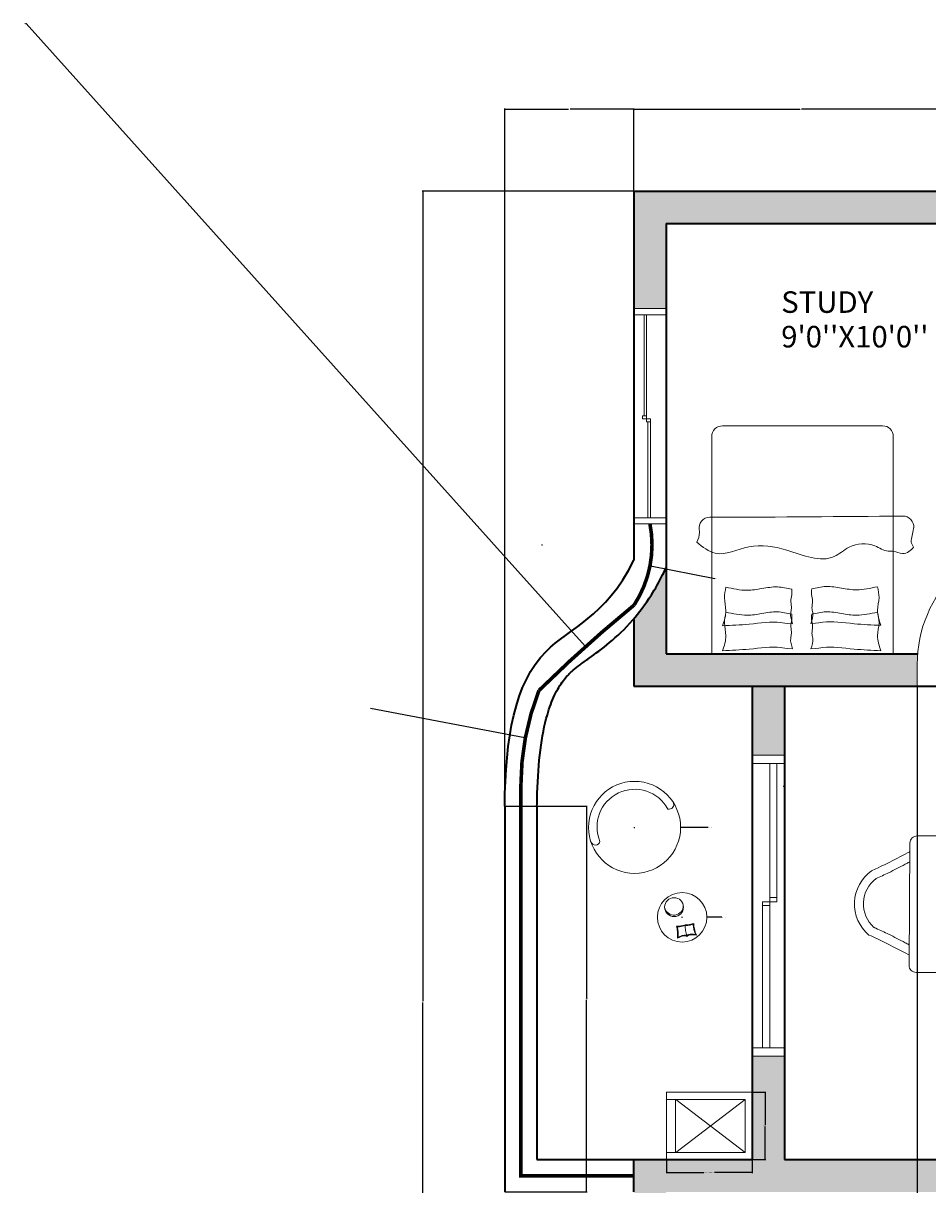
# Model space of a CAD drawing. Units: inches. Extents: x 1789 to 2841, y 3180 to 3702.
# Tile 2 of 14: x 1789 to 2041, y 3378 to 3702. Entities that reach past the tile are written whole.
import ezdxf

# ---------------------------------------------------------------- set-up
doc = ezdxf.new("R2010")
doc.units = ezdxf.units.IN
doc.header["$MEASUREMENT"] = 0
for name, color, linetype, lineweight in [('A-ANNO-DIMS', 2, 'Continuous', 18), ('A-AREA-IDEN', 7, 'Continuous', 18), ('A-FLOR-HRAL', 40, 'Continuous', 18), ('A-WALL', 40, 'Continuous', 35), ('A-WALL-PATT', 252, 'Continuous', 13), ('DORS', 70, 'Continuous', 18), ('FURNITURE', 34, 'Continuous', 18), ('WINDOWS', 130, 'Continuous', 18)]:
    doc.layers.add(name, color=color, linetype=linetype, lineweight=lineweight)
doc.styles.get("Standard").update_dxf_attribs({"font": 'arial.ttf'})
doc.dimstyles.get("Standard").update_dxf_attribs({"dimtxt": 0.18, "dimasz": 0.18, "dimexe": 0.18, "dimexo": 0.0625, "dimgap": 0.09, "dimtad": 0, "dimtih": 1, "dimtoh": 1, "dimdec": 0, "dimzin": 0, "dimdsep": 46, "dimlunit": 3, "dimtxsty": 'Standard', "dimcen": 0.09, "dimadec": 0, "dimazin": 0, "dimtfac": 1, "dimtdec": 0, "dimtofl": 0, "dimtmove": 0, "dimatfit": 3, "dimfxl": 1, "dimtolj": 1, "dimtzin": 0, "dimarcsym": 0})

# ---------------------------------------------------------------- blocks, each defined once
blk = doc.blocks.new('HYJ')
for p, q in [((2206.12, 3649.67), (2234.3, 3649.67)), ((2236.02, 3650.77), (2262.74, 3650.77)), ((2236.02, 3650.11), (2262.74, 3650.11)), ((2206.12, 3649), (2234.3, 3649))]:
    blk.add_line(p, q)
for points in [[(2204.43, 3646.16), (2264.43, 3646.16), (2264.43, 3655.16), (2204.43, 3655.16)], [(2204.43, 3655.16), (2206.12, 3655.16), (2206.12, 3646.16), (2204.43, 3646.16)], [(2264.43, 3655.16), (2262.74, 3655.16), (2262.74, 3646.16), (2264.43, 3646.16)], [(2234.3, 3649.67), (2235.16, 3649.67), (2235.16, 3648.56), (2234.3, 3648.56)], [(2235.16, 3650.77), (2236.02, 3650.77), (2236.02, 3649.67), (2235.16, 3649.67)]]:
    blk.add_lwpolyline(points, close=True)
blk = doc.blocks.new('BED')
blk.add_lwpolyline([(1986.04, 3526.16), (2036.66, 3526.16), (2036.66, 3586.73, 0.414214), (2033.66, 3589.73), (1989.04, 3589.73, 0.414214), (1986.04, 3586.73)], format="xyb", close=True)
for centre, start, end in [((1985.49, 3561.26), 90.0009, 190.5913), ((2039.35, 3561.59), 353.8505, 90.5407)]:
    blk.add_arc(centre, 3, start, end)
for points, knots in [([(1985.49, 3564.26), (1986.18, 3564.26), (2004.12, 3564.26), (2022.07, 3564.42), (2039.32, 3564.59)], [3.01567, 3.01567, 3.01567, 3.01567, 5.086115, 56.845422, 56.845422, 56.845422, 56.845422]), ([(1981.86, 3557.29), (1982.25, 3558.19), (1982.74, 3559.32), (1982.58, 3560.48), (1982.54, 3560.71)], [0, 0, 0, 0, 2.832176, 3.533558, 3.533558, 3.533558, 3.533558]), ([(2042.33, 3561.27), (2042.32, 3561.2), (2042.24, 3560.49), (2041.94, 3559.24), (2041.44, 3557.42), (2042.02, 3556.4), (2042.31, 3555.9)], [3.346066, 3.346066, 3.346066, 3.346066, 3.533964, 5.519604, 7.243879, 8.905148, 8.905148, 8.905148, 8.905148]), ([(1981.86, 3557.29), (1983.51, 3555.96), (1987.81, 3552.49), (1996.85, 3557.26), (2007.63, 3555.42), (2018.15, 3550.73), (2024.7, 3556.86), (2030.75, 3557.33), (2034.33, 3554.54), (2037.1, 3554.97), (2038.94, 3553.79), (2041.09, 3554.56), (2041.91, 3555.46), (2042.31, 3555.9)], [0, 0, 0, 0, 5.964303, 15.522281, 26.165437, 39.489609, 44.417923, 51.588888, 55.595283, 57.020157, 59.675402, 61.528396, 63.30469, 63.30469, 63.30469, 63.30469]), ([(1989.08, 3534), (1989.54, 3535.4), (1990.39, 3537.95), (1989.29, 3541.59), (1989.78, 3543.76), (1990, 3544.76)], [0, 0, 0, 0, 4.309756, 7.868817, 10.904955, 10.904955, 10.904955, 10.904955]), ([(1990, 3544.76), (1991.96, 3544.32), (1995.28, 3543.58), (2000.08, 3544.36), (2004.25, 3545.12), (2007.01, 3544.48), (2008.32, 3544.17)], [0, 0, 0, 0, 5.938346, 10.092725, 14.493934, 18.489388, 18.489388, 18.489388, 18.489388]), ([(2008.32, 3544.17), (2008.36, 3543.66), (2008.45, 3542.49), (2007.91, 3540.73), (2008.43, 3539.01), (2007.78, 3536.97), (2008.25, 3535.55), (2008.59, 3534.55)], [0, 0, 0, 0, 1.551238, 3.49035, 5.35792, 6.678685, 9.712273, 9.712273, 9.712273, 9.712273]), ([(2013.92, 3544.29), (2013.88, 3543.77), (2013.79, 3542.61), (2014.33, 3540.84), (2013.81, 3539.13), (2014.46, 3537.09), (2013.99, 3535.66), (2013.65, 3534.67)], [0, 0, 0, 0, 1.551238, 3.49035, 5.35792, 6.678685, 9.712273, 9.712273, 9.712273, 9.712273]), ([(2032.24, 3544.88), (2030.28, 3544.44), (2026.96, 3543.7), (2022.16, 3544.48), (2017.99, 3545.23), (2015.23, 3544.59), (2013.92, 3544.29)], [0, 0, 0, 0, 5.938346, 10.092725, 14.493934, 18.489388, 18.489388, 18.489388, 18.489388]), ([(2033.16, 3534.12), (2032.7, 3535.52), (2031.85, 3538.07), (2032.95, 3541.7), (2032.46, 3543.88), (2032.24, 3544.88)], [0, 0, 0, 0, 4.309756, 7.868817, 10.904955, 10.904955, 10.904955, 10.904955]), ([(1989.08, 3527.05), (1989.54, 3528.44), (1990.39, 3531), (1989.29, 3534.63), (1989.78, 3536.8), (1990, 3537.8)], [0, 0, 0, 0, 4.309756, 7.868817, 10.904955, 10.904955, 10.904955, 10.904955]), ([(1990, 3537.8), (1991.96, 3537.37), (1995.28, 3536.62), (2000.08, 3537.4), (2004.25, 3538.16), (2007.01, 3537.52), (2008.32, 3537.22)], [0, 0, 0, 0, 5.938346, 10.092725, 14.493934, 18.489388, 18.489388, 18.489388, 18.489388]), ([(2008.32, 3537.22), (2008.36, 3536.7), (2008.45, 3535.53), (2007.91, 3533.77), (2008.43, 3532.06), (2007.78, 3530.02), (2008.25, 3528.59), (2008.59, 3527.59)], [0, 0, 0, 0, 1.551238, 3.49035, 5.35792, 6.678685, 9.712273, 9.712273, 9.712273, 9.712273]), ([(2013.92, 3537.22), (2013.88, 3536.7), (2013.79, 3535.53), (2014.33, 3533.77), (2013.81, 3532.06), (2014.46, 3530.02), (2013.99, 3528.59), (2013.65, 3527.59)], [0, 0, 0, 0, 1.551238, 3.49035, 5.35792, 6.678685, 9.712273, 9.712273, 9.712273, 9.712273]), ([(2032.24, 3537.8), (2030.28, 3537.37), (2026.96, 3536.62), (2022.16, 3537.4), (2017.99, 3538.16), (2015.23, 3537.52), (2013.92, 3537.22)], [0, 0, 0, 0, 5.938346, 10.092725, 14.493934, 18.489388, 18.489388, 18.489388, 18.489388]), ([(2033.16, 3527.05), (2032.7, 3528.44), (2031.85, 3531), (2032.95, 3534.63), (2032.46, 3536.8), (2032.24, 3537.8)], [0, 0, 0, 0, 4.309756, 7.868817, 10.904955, 10.904955, 10.904955, 10.904955]), ([(1989.08, 3534), (1991.55, 3534.11), (1997.16, 3534.35), (2003.38, 3535.37), (2006.53, 3534.65), (2008.59, 3534.55)], [0, 0, 0, 0, 7.448152, 16.876341, 19.223863, 19.223863, 19.223863, 19.223863]), ([(2033.16, 3534.12), (2030.69, 3534.22), (2025.08, 3534.46), (2018.86, 3535.49), (2015.71, 3534.77), (2013.65, 3534.67)], [0, 0, 0, 0, 7.448152, 16.876341, 19.223863, 19.223863, 19.223863, 19.223863]), ([(1989.08, 3527.05), (1991.55, 3527.15), (1997.16, 3527.39), (2003.38, 3528.41), (2006.53, 3527.69), (2008.59, 3527.59)], [0, 0, 0, 0, 7.448152, 16.876341, 19.223863, 19.223863, 19.223863, 19.223863]), ([(2033.16, 3527.05), (2030.69, 3527.15), (2025.08, 3527.39), (2018.86, 3528.41), (2015.71, 3527.69), (2013.65, 3527.59)], [0, 0, 0, 0, 7.448152, 16.876341, 19.223863, 19.223863, 19.223863, 19.223863])]:
    blk.add_open_spline(points, degree=3, knots=knots)
blk = doc.blocks.new('*U9')
for p, q in [((0, 0), (0, -6)), ((36, 0), (36, -6))]:
    blk.add_line(p, q)
blk.add_lwpolyline([(0, 0), (0, 36), (1.75, 36), (1.75, 0)], close=True)
blk.add_arc((0, 0), 36, 0, 90)
blk = doc.blocks.new('WINDOW')
for p, q in [((1997.14, 3495.61), (1997.14, 3458.2)), ((1999.14, 3495.61), (1999.14, 3458.2)), ((1995.14, 3457.08), (1995.14, 3416.32)), ((1997.14, 3457.08), (1997.14, 3416.32))]:
    blk.add_line(p, q)
for points in [[(1992.23, 3497.95), (2001.23, 3497.95), (2001.23, 3413.99), (1992.23, 3413.99)], [(1992.23, 3497.95), (2001.23, 3497.95), (2001.23, 3495.61), (1992.23, 3495.61)], [(1995.14, 3455.97), (1997.14, 3455.97), (1997.14, 3457.08), (1995.14, 3457.08)], [(1997.14, 3457.08), (1999.14, 3457.08), (1999.14, 3458.2), (1997.14, 3458.2)], [(1992.23, 3413.99), (2001.23, 3413.99), (2001.23, 3416.32), (1992.23, 3416.32)]]:
    blk.add_lwpolyline(points, close=True)
blk = doc.blocks.new('DINI')
blk.add_lwpolyline([(2038.22, 3475.42), (2115.97, 3475.42, -0.414214), (2117.97, 3473.42), (2117.72, 3439.35, -0.414214), (2115.72, 3437.35), (2037.97, 3437.35, -0.414214), (2035.97, 3439.35), (2036.22, 3473.42, -0.414214)], format="xyb", close=True)
for centre, radius, start, end in [((2060.43, 3479.31), 11.31, 35.4017, 140.0736), ((2060.43, 3479.31), 8.8, 36.8657, 137.9611), ((2093.76, 3479.31), 11.31, 39.9264, 144.5983), ((2093.76, 3479.31), 8.8, 42.0389, 143.1343), ((2032.05, 3456.46), 11.31, 125.4017, 230.0736), ((2121.64, 3456.46), 11.31, 309.9264, 54.5983), ((2032.05, 3456.46), 8.8, 126.8657, 227.9611), ((2121.64, 3456.46), 8.8, 312.0389, 53.1343), ((2060.43, 3433.45), 11.31, 219.9264, 324.5983), ((2060.43, 3433.45), 8.8, 222.0389, 323.1343), ((2093.76, 3433.45), 11.31, 215.4017, 320.0736), ((2093.76, 3433.45), 8.8, 216.8657, 317.9611)]:
    blk.add_arc(centre, radius, start, end)
for points, knots in [([(2046.22, 3475.42), (2047.75, 3478.33), (2049.68, 3482.01), (2051.4, 3485.79), (2051.76, 3486.58)], [0, 0, 0, 0, 7.856931, 9.915256, 9.915256, 9.915256, 9.915256]), ([(2049.05, 3475.42), (2049.25, 3475.79), (2049.44, 3476.15), (2050.42, 3478.03), (2051.21, 3479.56), (2052.54, 3482.27), (2053.1, 3483.45), (2053.72, 3484.82), (2053.81, 3485.01), (2053.9, 3485.21)], [1.048693, 1.048693, 1.048693, 1.048693, 2.029233, 2.029233, 6.0877, 6.0877, 9.118148, 9.118148, 9.624349, 9.624349, 9.624349, 9.624349]), ([(2072.04, 3475.42), (2071.85, 3475.78), (2071.66, 3476.15), (2070.68, 3478.03), (2069.89, 3479.55), (2068.56, 3482.26), (2068.01, 3483.43), (2067.48, 3484.59)], [1.048889, 1.048889, 1.048889, 1.048889, 2.02655, 2.02655, 6.079649, 6.079649, 9.095857, 9.095857, 9.095857, 9.095857]), ([(2074.88, 3475.42), (2073.35, 3478.33), (2071.54, 3481.78), (2069.91, 3485.32), (2069.66, 3485.87)], [0, 0, 0, 0, 7.856931, 9.297576, 9.297576, 9.297576, 9.297576]), ([(2079.31, 3475.42), (2080.85, 3478.33), (2082.66, 3481.78), (2084.29, 3485.32), (2084.54, 3485.87)], [0, 0, 0, 0, 7.856931, 9.297576, 9.297576, 9.297576, 9.297576]), ([(2082.15, 3475.42), (2082.34, 3475.78), (2082.53, 3476.15), (2083.51, 3478.03), (2084.3, 3479.55), (2085.63, 3482.26), (2086.19, 3483.43), (2086.72, 3484.59)], [1.048889, 1.048889, 1.048889, 1.048889, 2.02655, 2.02655, 6.079649, 6.079649, 9.095857, 9.095857, 9.095857, 9.095857]), ([(2105.14, 3475.42), (2104.95, 3475.79), (2104.76, 3476.15), (2103.78, 3478.03), (2102.99, 3479.56), (2101.65, 3482.27), (2101.1, 3483.45), (2100.47, 3484.82), (2100.38, 3485.01), (2100.3, 3485.21)], [1.048693, 1.048693, 1.048693, 1.048693, 2.029233, 2.029233, 6.0877, 6.0877, 9.118148, 9.118148, 9.624349, 9.624349, 9.624349, 9.624349]), ([(2107.98, 3475.42), (2106.45, 3478.33), (2104.51, 3482.01), (2102.79, 3485.79), (2102.44, 3486.58)], [0, 0, 0, 0, 7.856931, 9.915256, 9.915256, 9.915256, 9.915256]), ([(2036.2, 3471.04), (2036.05, 3470.96), (2035.89, 3470.88), (2035.74, 3470.8), (2035.74, 3470.8), (2035.74, 3470.8), (2035.74, 3470.8), (2032.89, 3469.3), (2029.51, 3467.53), (2026.05, 3465.93), (2025.5, 3465.68)], [-0.229823, -0.229823, -0.229823, -0.229823, 0.189373, 0.189373, 0.189373, 0.189712, 0.189712, 0.189712, 7.856931, 9.297576, 9.297576, 9.297576, 9.297576]), ([(2036.18, 3468.19), (2036.04, 3468.12), (2035.9, 3468.04), (2035.76, 3467.97), (2035.76, 3467.97), (2035.76, 3467.97), (2035.76, 3467.97), (2035.46, 3467.81), (2035.16, 3467.65), (2033.34, 3466.71), (2031.81, 3465.92), (2029.11, 3464.59), (2027.94, 3464.04), (2026.77, 3463.5)], [0.838882, 0.838882, 0.838882, 0.838882, 1.215073, 1.215073, 1.215073, 1.219193, 1.219193, 1.219193, 2.02655, 2.02655, 6.079649, 6.079649, 9.095857, 9.095857, 9.095857, 9.095857]), ([(2117.95, 3470.8), (2120.8, 3469.3), (2124.18, 3467.53), (2127.64, 3465.93), (2128.19, 3465.68)], [0.189712, 0.189712, 0.189712, 0.189712, 7.856931, 9.297576, 9.297576, 9.297576, 9.297576]), ([(2117.93, 3467.97), (2118.23, 3467.81), (2118.53, 3467.65), (2120.35, 3466.71), (2121.88, 3465.92), (2124.58, 3464.59), (2125.75, 3464.04), (2126.92, 3463.5)], [1.219193, 1.219193, 1.219193, 1.219193, 2.02655, 2.02655, 6.079649, 6.079649, 9.095857, 9.095857, 9.095857, 9.095857]), ([(2035.95, 3445.08), (2035.58, 3445.27), (2035.22, 3445.46), (2033.34, 3446.45), (2031.81, 3447.23), (2029.1, 3448.57), (2027.92, 3449.12), (2026.55, 3449.75), (2026.36, 3449.84), (2026.16, 3449.93)], [1.048693, 1.048693, 1.048693, 1.048693, 2.029233, 2.029233, 6.0877, 6.0877, 9.118148, 9.118148, 9.624349, 9.624349, 9.624349, 9.624349]), ([(2117.74, 3445.08), (2118.11, 3445.27), (2118.47, 3445.46), (2120.35, 3446.45), (2121.88, 3447.23), (2124.59, 3448.57), (2125.77, 3449.12), (2127.14, 3449.75), (2127.33, 3449.84), (2127.53, 3449.93)], [1.048693, 1.048693, 1.048693, 1.048693, 2.029233, 2.029233, 6.0877, 6.0877, 9.118148, 9.118148, 9.624349, 9.624349, 9.624349, 9.624349]), ([(2035.95, 3442.24), (2033.03, 3443.77), (2029.36, 3445.71), (2025.58, 3447.43), (2024.79, 3447.79)], [0, 0, 0, 0, 7.856931, 9.915256, 9.915256, 9.915256, 9.915256]), ([(2117.74, 3442.24), (2120.66, 3443.77), (2124.33, 3445.71), (2128.11, 3447.43), (2128.9, 3447.79)], [0, 0, 0, 0, 7.856931, 9.915256, 9.915256, 9.915256, 9.915256]), ([(2046.22, 3437.35), (2047.75, 3434.43), (2049.68, 3430.75), (2051.4, 3426.98), (2051.76, 3426.19)], [0, 0, 0, 0, 7.856931, 9.915256, 9.915256, 9.915256, 9.915256]), ([(2049.05, 3437.35), (2049.25, 3436.98), (2049.44, 3436.62), (2050.42, 3434.73), (2051.21, 3433.2), (2052.54, 3430.5), (2053.1, 3429.32), (2053.72, 3427.95), (2053.81, 3427.75), (2053.9, 3427.56)], [1.048693, 1.048693, 1.048693, 1.048693, 2.029233, 2.029233, 6.0877, 6.0877, 9.118148, 9.118148, 9.624349, 9.624349, 9.624349, 9.624349]), ([(2072.04, 3437.35), (2071.85, 3436.98), (2071.66, 3436.62), (2070.68, 3434.74), (2069.89, 3433.21), (2068.56, 3430.51), (2068.01, 3429.34), (2067.48, 3428.17)], [1.048889, 1.048889, 1.048889, 1.048889, 2.02655, 2.02655, 6.079649, 6.079649, 9.095857, 9.095857, 9.095857, 9.095857]), ([(2074.88, 3437.35), (2073.35, 3434.43), (2071.54, 3430.98), (2069.91, 3427.45), (2069.66, 3426.9)], [0, 0, 0, 0, 7.856931, 9.297576, 9.297576, 9.297576, 9.297576]), ([(2079.31, 3437.35), (2080.85, 3434.43), (2082.66, 3430.98), (2084.29, 3427.45), (2084.54, 3426.9)], [0, 0, 0, 0, 7.856931, 9.297576, 9.297576, 9.297576, 9.297576]), ([(2082.15, 3437.35), (2082.34, 3436.98), (2082.53, 3436.62), (2083.51, 3434.74), (2084.3, 3433.21), (2085.63, 3430.51), (2086.19, 3429.34), (2086.72, 3428.17)], [1.048889, 1.048889, 1.048889, 1.048889, 2.02655, 2.02655, 6.079649, 6.079649, 9.095857, 9.095857, 9.095857, 9.095857]), ([(2105.14, 3437.35), (2104.95, 3436.98), (2104.76, 3436.62), (2103.78, 3434.73), (2102.99, 3433.2), (2101.65, 3430.5), (2101.1, 3429.32), (2100.47, 3427.95), (2100.38, 3427.75), (2100.3, 3427.56)], [1.048693, 1.048693, 1.048693, 1.048693, 2.029233, 2.029233, 6.0877, 6.0877, 9.118148, 9.118148, 9.624349, 9.624349, 9.624349, 9.624349]), ([(2107.98, 3437.35), (2106.45, 3434.43), (2104.51, 3430.75), (2102.79, 3426.98), (2102.44, 3426.19)], [0, 0, 0, 0, 7.856931, 9.915256, 9.915256, 9.915256, 9.915256])]:
    blk.add_open_spline(points, degree=3, knots=knots)
blk = doc.blocks.new('GTGTGTGT')
for p, q in [((1970.85, 3401.93), (1970.85, 3387.16)), ((1970.92, 3401.93), (1990.23, 3387.16)), ((1970.92, 3387.16), (1990.23, 3401.93))]:
    blk.add_line(p, q)
for points in [[(1992.23, 3385.16), (1968.3, 3385.16), (1968.3, 3403.93), (1992.23, 3403.93)], [(1990.23, 3387.16), (1968.3, 3387.16), (1968.3, 3401.93), (1990.23, 3401.93)]]:
    blk.add_lwpolyline(points, close=True)
blk = doc.blocks.new('*D73')
at = {"layer": 'A-ANNO-DIMS', "color": 0, "lineweight": -2, "transparency": 16777216}
for p, q in [((1968.3, 3385.1), (1968.3, 3381.39)), ((1992.23, 3385.1), (1992.23, 3381.39)), ((1968.48, 3381.57), (1978.78, 3381.57)), ((1992.05, 3381.57), (1981.76, 3381.57))]:
    blk.add_line(p, q, dxfattribs=at)
at = {"layer": 'A-ANNO-DIMS', "color": 0, "transparency": 16777216}
for points in [[(1968.48, 3381.6), (1968.48, 3381.54), (1968.3, 3381.57)], [(1992.05, 3381.6), (1992.05, 3381.54), (1992.23, 3381.57)]]:
    blk.add_solid(points, dxfattribs=at)
at = {"layer": 'Defpoints', "color": 0, "transparency": 16777216}
for p in [(1968.3, 3385.16), (1992.23, 3385.16), (1992.23, 3381.57)]:
    blk.add_point(p, dxfattribs=at)
at = {"layer": 'A-ANNO-DIMS', "color": 0, "transparency": 16777216, "insert": (1980.27, 3381.57), "char_height": 0.18, "attachment_point": 5}
blk.add_mtext('\\A1;BALCONY UNIT 24 TYP.', dxfattribs=at)
blk = doc.blocks.new('*D74')
at = {"layer": 'A-ANNO-DIMS', "color": 0, "lineweight": -2, "transparency": 16777216}
for p, q in [((1992.3, 3403.93), (1996, 3403.93)), ((1995.82, 3403.75), (1995.82, 3394.73)), ((1995.82, 3385.34), (1995.82, 3394.37)), ((1992.3, 3385.16), (1996, 3385.16))]:
    blk.add_line(p, q, dxfattribs=at)
at = {"layer": 'A-ANNO-DIMS', "color": 0, "transparency": 16777216}
for points in [[(1995.79, 3403.75), (1995.85, 3403.75), (1995.82, 3403.93)], [(1995.79, 3385.34), (1995.85, 3385.34), (1995.82, 3385.16)]]:
    blk.add_solid(points, dxfattribs=at)
at = {"layer": 'Defpoints', "color": 0, "transparency": 16777216}
for p in [(1992.23, 3403.93), (1995.82, 3403.93), (1992.23, 3385.16)]:
    blk.add_point(p, dxfattribs=at)
at = {"layer": 'A-ANNO-DIMS', "color": 0, "transparency": 16777216, "insert": (1995.82, 3394.55), "char_height": 0.18, "attachment_point": 5}
blk.add_mtext('\\A1;19 TYP.', dxfattribs=at)
blk = doc.blocks.new('*D80')
at = {"layer": 'A-ANNO-DIMS', "color": 0, "lineweight": -2, "transparency": 16777216}
for p, q in [((1959.17, 3655.16), (1900.2, 3655.16)), ((1900.38, 3654.98), (1900.38, 3429.34)), ((1900.38, 3203.34), (1900.38, 3428.98)), ((1959.17, 3203.16), (1900.2, 3203.16))]:
    blk.add_line(p, q, dxfattribs=at)
at = {"layer": 'A-ANNO-DIMS', "color": 0, "transparency": 16777216}
for points in [[(1900.35, 3654.98), (1900.41, 3654.98), (1900.38, 3655.16)], [(1900.35, 3203.34), (1900.41, 3203.34), (1900.38, 3203.16)]]:
    blk.add_solid(points, dxfattribs=at)
at = {"layer": 'Defpoints', "color": 0, "transparency": 16777216}
for p in [(1959.23, 3655.16), (1900.38, 3203.16), (1959.23, 3203.16)]:
    blk.add_point(p, dxfattribs=at)
at = {"layer": 'A-ANNO-DIMS', "color": 0, "transparency": 16777216, "insert": (1900.38, 3429.16), "char_height": 0.18, "attachment_point": 5}
blk.add_mtext('\\A1;452', dxfattribs=at)
blk = doc.blocks.new('*D81')
at = {"layer": 'A-ANNO-DIMS', "color": 0, "lineweight": -2, "transparency": 16777216}
for p, q in [((1923.23, 3483.75), (1923.23, 3678.19)), ((1923.41, 3678.01), (1941.01, 3678.01)), ((1959.05, 3678.01), (1941.45, 3678.01)), ((1959.23, 3655.22), (1959.23, 3678.19))]:
    blk.add_line(p, q, dxfattribs=at)
at = {"layer": 'A-ANNO-DIMS', "color": 0, "transparency": 16777216}
for points in [[(1923.41, 3678.04), (1923.41, 3677.98), (1923.23, 3678.01)], [(1959.05, 3678.04), (1959.05, 3677.98), (1959.23, 3678.01)]]:
    blk.add_solid(points, dxfattribs=at)
at = {"layer": 'Defpoints', "color": 0, "transparency": 16777216}
for p in [(1959.23, 3678.01), (1959.23, 3655.16), (1923.23, 3483.69)]:
    blk.add_point(p, dxfattribs=at)
at = {"layer": 'A-ANNO-DIMS', "color": 0, "transparency": 16777216, "insert": (1941.23, 3678.01), "char_height": 0.18, "attachment_point": 5}
blk.add_mtext('\\A1;36', dxfattribs=at)
blk = doc.blocks.new('*D82')
at = {"layer": 'A-ANNO-DIMS', "color": 0, "lineweight": -2, "transparency": 16777216}
for p, q in [((1959.23, 3655.22), (1959.23, 3678.19)), ((1959.41, 3678.01), (2005.51, 3678.01)), ((2052.05, 3678.01), (2005.95, 3678.01)), ((2052.23, 3655.22), (2052.23, 3678.19))]:
    blk.add_line(p, q, dxfattribs=at)
at = {"layer": 'A-ANNO-DIMS', "color": 0, "transparency": 16777216}
for points in [[(1959.41, 3678.04), (1959.41, 3677.98), (1959.23, 3678.01)], [(2052.05, 3678.04), (2052.05, 3677.98), (2052.23, 3678.01)]]:
    blk.add_solid(points, dxfattribs=at)
at = {"layer": 'Defpoints', "color": 0, "transparency": 16777216}
for p in [(2052.23, 3678.01), (1959.23, 3655.16), (2052.23, 3655.16)]:
    blk.add_point(p, dxfattribs=at)
at = {"layer": 'A-ANNO-DIMS', "color": 0, "transparency": 16777216, "insert": (2005.73, 3678.01), "char_height": 0.18, "attachment_point": 5}
blk.add_mtext('\\A1;93', dxfattribs=at)
blk = doc.blocks.new('*D90')
at = {"layer": 'A-ANNO-DIMS', "color": 0, "lineweight": -2, "transparency": 16777216}
for p, q in [((2038.23, 3517.1), (2038.23, 3180.13)), ((2074.23, 3517.1), (2074.23, 3180.13)), ((2038.41, 3180.31), (2056.01, 3180.31)), ((2074.05, 3180.31), (2056.45, 3180.31))]:
    blk.add_line(p, q, dxfattribs=at)
at = {"layer": 'A-ANNO-DIMS', "color": 0, "transparency": 16777216}
for points in [[(2038.41, 3180.34), (2038.41, 3180.28), (2038.23, 3180.31)], [(2074.05, 3180.34), (2074.05, 3180.28), (2074.23, 3180.31)]]:
    blk.add_solid(points, dxfattribs=at)
at = {"layer": 'Defpoints', "color": 0, "transparency": 16777216}
for p in [(2038.23, 3517.16), (2074.23, 3517.16), (2074.23, 3180.31)]:
    blk.add_point(p, dxfattribs=at)
at = {"layer": 'A-ANNO-DIMS', "color": 0, "transparency": 16777216, "insert": (2056.23, 3180.31), "char_height": 0.18, "attachment_point": 5}
blk.add_mtext('\\A1;36', dxfattribs=at)
blk = doc.blocks.new('*D94')
at = {"layer": 'A-ANNO-DIMS', "color": 0, "lineweight": -2, "transparency": 16777216}
for p, q in [((1923.3, 3483.69), (1946.26, 3483.69)), ((1946.08, 3483.51), (1946.08, 3430.11)), ((1946.08, 3376.34), (1946.08, 3429.74)), ((1923.3, 3376.16), (1946.26, 3376.16))]:
    blk.add_line(p, q, dxfattribs=at)
at = {"layer": 'A-ANNO-DIMS', "color": 0, "transparency": 16777216}
for points in [[(1946.05, 3483.51), (1946.11, 3483.51), (1946.08, 3483.69)], [(1946.05, 3376.34), (1946.11, 3376.34), (1946.08, 3376.16)]]:
    blk.add_solid(points, dxfattribs=at)
at = {"layer": 'Defpoints', "color": 0, "transparency": 16777216}
for p in [(1923.23, 3483.69), (1923.23, 3376.16), (1946.08, 3376.16)]:
    blk.add_point(p, dxfattribs=at)
at = {"layer": 'A-ANNO-DIMS', "color": 0, "transparency": 16777216, "insert": (1946.08, 3429.92), "char_height": 0.18, "attachment_point": 5}
blk.add_mtext('\\A1;107.53', dxfattribs=at)
blk = doc.blocks.new('*D115')
at = {"layer": 'A-ANNO-DIMS', "color": 0, "lineweight": -2, "transparency": 16777216}
for p, q in [((1885.79, 3510.98), (1928.83, 3502.86)), ((2000.93, 3489.24), (2001.11, 3489.24)), ((2001.02, 3489.15), (2001.02, 3489.33))]:
    blk.add_line(p, q, dxfattribs=at)
at = {"layer": 'A-ANNO-DIMS', "color": 0, "transparency": 16777216}
blk.add_solid([(1928.83, 3502.89), (1928.82, 3502.83), (1929, 3502.83)], dxfattribs=at)
at = {"layer": 'Defpoints', "color": 0, "transparency": 16777216}
for p in [(1929, 3502.83), (2001.02, 3489.24)]:
    blk.add_point(p, dxfattribs=at)
at = {"layer": 'A-ANNO-DIMS', "color": 0, "transparency": 16777216, "insert": (1885.31, 3510.98), "char_height": 0.18, "attachment_point": 5}
blk.add_mtext('\\A1;R73.29', dxfattribs=at)
blk = doc.blocks.new('*D116')
at = {"layer": 'A-ANNO-DIMS', "color": 0, "lineweight": -2, "transparency": 16777216}
for p, q in [((1789.65, 3701.85), (1789.83, 3701.85)), ((1789.83, 3701.85), (1945.65, 3528.3)), ((2205.56, 3238.68), (2205.74, 3238.68)), ((2205.65, 3238.59), (2205.65, 3238.77))]:
    blk.add_line(p, q, dxfattribs=at)
at = {"layer": 'A-ANNO-DIMS', "color": 0, "transparency": 16777216}
blk.add_solid([(1945.67, 3528.32), (1945.62, 3528.28), (1945.77, 3528.16)], dxfattribs=at)
at = {"layer": 'Defpoints', "color": 0, "transparency": 16777216}
for p in [(1945.77, 3528.16), (2205.65, 3238.68)]:
    blk.add_point(p, dxfattribs=at)
at = {"layer": 'A-ANNO-DIMS', "color": 0, "transparency": 16777216, "insert": (1789.28, 3701.85), "char_height": 0.18, "attachment_point": 5}
blk.add_mtext('\\A1;R389', dxfattribs=at)
blk = doc.blocks.new('*D117')
at = {"layer": 'A-ANNO-DIMS', "color": 0, "lineweight": -2, "transparency": 16777216}
for p, q in [((1933.56, 3556.53), (1933.74, 3556.53)), ((1933.65, 3556.44), (1933.65, 3556.62)), ((1981.78, 3547.12), (1963.91, 3550.62))]:
    blk.add_line(p, q, dxfattribs=at)
at = {"layer": 'A-ANNO-DIMS', "color": 0, "transparency": 16777216}
blk.add_solid([(1963.91, 3550.64), (1963.9, 3550.59), (1963.73, 3550.65)], dxfattribs=at)
at = {"layer": 'Defpoints', "color": 0, "transparency": 16777216}
for p in [(1933.65, 3556.53), (1963.73, 3550.65)]:
    blk.add_point(p, dxfattribs=at)
at = {"layer": 'A-ANNO-DIMS', "color": 0, "transparency": 16777216, "insert": (1982.26, 3547.12), "char_height": 0.18, "attachment_point": 5}
blk.add_mtext('\\A1;R30.65', dxfattribs=at)
blk = doc.blocks.new('*D118')
at = {"layer": 'A-ANNO-DIMS', "color": 0, "lineweight": -2, "transparency": 16777216}
for p, q in [((1959.36, 3477.79), (1959.54, 3477.79)), ((1959.45, 3477.7), (1959.45, 3477.88)), ((1979.97, 3477.79), (1972.46, 3477.79))]:
    blk.add_line(p, q, dxfattribs=at)
at = {"layer": 'A-ANNO-DIMS', "color": 0, "transparency": 16777216}
blk.add_solid([(1972.46, 3477.82), (1972.46, 3477.76), (1972.28, 3477.79)], dxfattribs=at)
at = {"layer": 'Defpoints', "color": 0, "transparency": 16777216}
for p in [(1946.61, 3477.79), (1972.28, 3477.79)]:
    blk.add_point(p, dxfattribs=at)
at = {"layer": 'A-ANNO-DIMS', "color": 0, "transparency": 16777216, "insert": (1980.47, 3477.79), "char_height": 0.18, "attachment_point": 5}
blk.add_mtext('\\A1;∅25.66', dxfattribs=at)
blk = doc.blocks.new('*D119')
at = {"layer": 'A-ANNO-DIMS', "color": 0, "lineweight": -2, "transparency": 16777216}
for p, q in [((1972.61, 3452.73), (1972.79, 3452.73)), ((1972.7, 3452.64), (1972.7, 3452.82)), ((1983.73, 3452.73), (1979.77, 3452.73))]:
    blk.add_line(p, q, dxfattribs=at)
at = {"layer": 'A-ANNO-DIMS', "color": 0, "transparency": 16777216}
blk.add_solid([(1979.77, 3452.76), (1979.77, 3452.7), (1979.59, 3452.73)], dxfattribs=at)
at = {"layer": 'Defpoints', "color": 0, "transparency": 16777216}
for p in [(1965.8, 3452.73), (1979.59, 3452.73)]:
    blk.add_point(p, dxfattribs=at)
at = {"layer": 'A-ANNO-DIMS', "color": 0, "transparency": 16777216, "insert": (1984.29, 3452.73), "char_height": 0.18, "attachment_point": 5}
blk.add_mtext('\\A1;∅13.788', dxfattribs=at)

msp = doc.modelspace()

# ---------------------------------------------------------------- hatches: boundary and pattern name
at = {"layer": 'A-WALL-PATT'}
h = msp.add_hatch(color=256, dxfattribs=at)
h.dxf.hatch_style = 1
h.paths.add_polyline_path([(2052.2333, 3646.1608), (2052.2333, 3655.1608), (1959.2333, 3655.1608), (1959.2333, 3622.3936), (1968.2333, 3622.3936), (1968.2333, 3646.1608)])
h.paths.add_polyline_path([(2163.2333, 3646.1608), (2163.2333, 3640.1475), (2163.2333, 3568.1608), (2159.2333, 3568.1608), (2159.2333, 3565.4274), (2163.2333, 3565.4274), (2163.2333, 3564.1608), (2169.2333, 3564.1608, -0.02086055), (2172.2333, 3564.0356), (2172.2333, 3646.1608), (2196.2333, 3646.1608), (2204.4325, 3646.1608), (2204.4325, 3655.1608), (2117.6786, 3655.1608), (2117.6786, 3646.1608)])
h.paths.add_polyline_path([(2085.2333, 3646.1608), (2093.6786, 3646.1608), (2093.6786, 3655.1608), (2076.2333, 3655.1608), (2076.2333, 3646.1608), (2076.2333, 3621.0865), (2076.2333, 3526.1608), (2074.2333, 3526.1608), (2074.2333, 3523.1608), (2074.2333, 3517.1608), (2085.2333, 3517.1608), (2085.2333, 3565.4274), (2129.2333, 3565.4274), (2129.2333, 3568.1608), (2085.2333, 3568.1608)])
h.paths.add_polyline_path([(2172.2333, 3526.1608), (2172.2333, 3528.1608), (2163.2333, 3528.1608), (2163.2333, 3517.1608), (2316.2333, 3517.1608), (2316.2333, 3513.1608), (2319.2333, 3513.1608), (2325.2333, 3513.1608), (2325.2333, 3584.2279), (2316.2333, 3584.2279), (2316.2333, 3526.1608)])
h.paths.add_polyline_path([(2325.2333, 3655.1608), (2264.4325, 3655.1608), (2264.4325, 3646.1608), (2316.2333, 3646.1608), (2316.2333, 3633.8369), (2316.2333, 3620.2279), (2325.2333, 3620.2279)])
h = msp.add_hatch(color=256, dxfattribs=at)
h.dxf.hatch_style = 1
edge = h.paths.add_edge_path()
edge.add_line((2038.2333, 3517.1608), (2038.2333, 3523.1608))
edge.add_arc((2074.2333, 3523.1608), 36, 175.219808, 180, ccw=False)
edge.add_line((2038.3586, 3526.1608), (1968.2333, 3526.1608))
edge.add_line((1968.2333, 3526.1608), (1968.2333, 3550.1092))
edge.add_spline(control_points=[(1968.2333, 3550.1092), (1967.93, 3549.5057), (1967.6267, 3548.9021), (1967.3234, 3548.2985), (1967.3062, 3548.2643), (1967.289, 3548.2301), (1967.2718, 3548.1959)], knot_values=[86.1489403, 86.1489403, 86.1489403, 86.1489403, 87.2957089, 87.2957089, 87.2957089, 87.36071802, 87.36071802, 87.36071802, 87.36071802], degree=3, periodic=0)
edge.add_spline(control_points=[(1967.2718, 3548.1959), (1966.2637, 3546.1938), (1965.2159, 3544.3437), (1962.5553, 3540.1233), (1960.9051, 3537.9117), (1959.2333, 3535.9585)], knot_values=[76.75836165, 76.75836165, 76.75836165, 76.75836165, 80.56743471, 80.56743471, 86.1489403, 86.1489403, 86.1489403, 86.1489403], degree=3, periodic=0)
edge.add_line((1959.2333, 3535.9585), (1959.2333, 3517.1608))
edge.add_line((1959.2333, 3517.1608), (2038.2333, 3517.1608))
h = msp.add_hatch(color=256, dxfattribs=at)
h.dxf.hatch_style = 1
h.paths.add_polyline_path([(2001.2333, 3517.1608), (1992.2333, 3517.1608), (1992.2333, 3497.9466), (2001.2333, 3497.9466)])
h = msp.add_hatch(color=256, dxfattribs=at)
h.dxf.hatch_style = 1
h.paths.add_polyline_path([(1968.2333, 3376.1608), (2072.0492, 3376.1608, -0.02086055), (2071.924, 3379.1608), (2071.924, 3385.1608), (2001.2333, 3385.1608), (2001.2333, 3413.9882), (1992.2333, 3413.9882), (1992.2333, 3385.1608), (1968.3016, 3385.1608), (1959.2333, 3385.1608), (1959.2333, 3376.1608), (1959.2333, 3260.1608), (1968.2333, 3260.1608), (1968.2333, 3275.5886), (1968.2333, 3332.3251)])

# ---------------------------------------------------------------- linework, layer by layer
at = {"layer": 'A-FLOR-HRAL', "const_width": 1}
msp.add_lwpolyline([(1959.2333, 3380.6608), (1927.7333, 3380.6608), (1927.7333, 3489.2423, -0.09351003), (1932.7716, 3515.9465, -0.02292859), (1959.3071, 3539.7695, 0.19519551), (1963.7333, 3562.3936, -22.61576082)], format="xyb", dxfattribs=at)
at = {"layer": 'A-WALL'}
for p, q in [((1959.2333, 3655.1608), (1959.2333, 3552.2435)), ((1959.2333, 3655.1608), (2325.2333, 3655.1608)), ((1968.2333, 3646.1608), (1968.2333, 3526.1608)), ((1968.2333, 3646.1608), (2076.2333, 3646.1608)), ((1959.2333, 3535.9585), (1959.2333, 3517.1608)), ((1968.2333, 3526.1608), (2038.3586, 3526.1608)), ((1959.2333, 3517.1608), (2085.2333, 3517.1608)), ((1992.2333, 3517.1608), (1992.2333, 3385.1608)), ((2001.2333, 3517.1608), (2001.2333, 3385.1608)), ((1923.2333, 3483.6885), (1923.2333, 3376.1608)), ((1932.2333, 3483.637), (1932.2333, 3385.1608)), ((1932.2333, 3385.1608), (1992.2333, 3385.1608)), ((1959.2333, 3376.1608), (1959.2333, 3385.1608)), ((2001.2333, 3385.1608), (2071.924, 3385.1608))]:
    msp.add_line(p, q, dxfattribs=at)
for points, knots in [([(1923.2333, 3483.6885), (1923.4364, 3502.604), (1927.8202, 3529.4244), (1951.1776, 3536.2446), (1959.2333, 3552.2435)], [4.35013907, 4.35013907, 4.35013907, 4.35013907, 51.40968685, 86.1489403, 86.1489403, 86.1489403, 86.1489403]), ([(1932.2333, 3483.637), (1932.247, 3484.8899), (1932.2713, 3486.122), (1932.4351, 3491.6434), (1932.7121, 3495.6714), (1933.6352, 3503.0125), (1934.2828, 3506.3237), (1935.7012, 3511.2214), (1936.3756, 3513.0265), (1937.8781, 3516.196), (1938.7038, 3517.5593), (1939.9903, 3519.2429), (1940.3954, 3519.7191), (1941.0419, 3520.4018), (1941.2692, 3520.6281), (1941.7671, 3521.0969), (1942.0345, 3521.336), (1942.8968, 3522.0728), (1943.5526, 3522.59), (1945.0276, 3523.6991), (1945.8464, 3524.2909), (1948.4351, 3526.1643), (1950.3942, 3527.5827), (1954.5642, 3531.0612), (1956.7702, 3533.1254), (1960.7158, 3537.6593), (1962.4647, 3539.9796), (1965.2159, 3544.3437), (1966.2637, 3546.1938), (1967.2718, 3548.1959), (1967.289, 3548.2301), (1967.3062, 3548.2643), (1967.3234, 3548.2985), (1967.6267, 3548.9021), (1967.93, 3549.5057), (1968.2333, 3550.1092)], [4.38907139, 4.38907139, 4.38907139, 4.38907139, 7.6358486, 7.6358486, 19.20888675, 19.20888675, 30.78192491, 30.78192491, 38.89033862, 38.89033862, 46.99875233, 46.99875233, 50.54541348, 50.54541348, 52.44307722, 52.44307722, 54.34074096, 54.34074096, 58.13606845, 58.13606845, 61.93139593, 61.93139593, 69.18500608, 69.18500608, 76.43861623, 76.43861623, 82.33986724, 82.33986724, 86.1489403, 86.1489403, 86.1489403, 86.21394942, 86.21394942, 86.21394942, 87.36071802, 87.36071802, 87.36071802, 87.36071802])]:
    msp.add_open_spline(points, degree=3, knots=knots, dxfattribs=at)
at = {"layer": 'FURNITURE'}
for centre, radius in [((1959.4452, 3477.7931), 12.831), ((1972.6953, 3452.7282), 6.8942), ((1970.4534, 3455.5625), 2.6277)]:
    msp.add_circle(centre, radius, dxfattribs=at)
for centre, radius, start, end in [((1959.4728, 3477.9116), 10.4983, 28.206792, 202.753412), ((1969.0378, 3484.1563), 1.3203, 256.270622, 31.893098), ((1948.514, 3474.1851), 1.3203, 199.931412, 345.655525), ((1970.4054, 3455.9695), 2.6277, 191.187475, 2.24156)]:
    msp.add_arc(centre, radius, start, end, dxfattribs=at)
for points, knots in [([(1971.0886, 3450.2504), (1971.634, 3450.2599), (1972.4613, 3450.2744), (1973.2476, 3450.5203), (1973.5155, 3450.604)], [0, 0, 0, 0, 1.62352899, 2.46269241, 2.46269241, 2.46269241, 2.46269241]), ([(1971.0886, 3450.2504), (1971.217, 3449.7489), (1971.4997, 3448.6452), (1971.4369, 3447.506), (1971.4026, 3446.8844)], [0, 0, 0, 0, 1.54412343, 3.39829197, 3.39829197, 3.39829197, 3.39829197]), ([(1971.308, 3450.0832), (1971.5181, 3450.0876), (1971.7294, 3450.0939), (1972.2397, 3450.1281), (1972.5404, 3450.1646), (1973.0856, 3450.29), (1973.3282, 3450.3661), (1973.5092, 3450.4331)], [0.12510297, 0.12510297, 0.12510297, 0.12510297, 0.48878032, 0.48878032, 1.00205856, 1.00205856, 1.43827739, 1.43827739, 1.43827739, 1.43827739]), ([(1971.308, 3450.0832), (1971.363, 3449.866), (1971.4165, 3449.6472), (1971.5387, 3449.0621), (1971.5903, 3448.6888), (1971.622, 3447.9436), (1971.6095, 3447.5716), (1971.5904, 3447.189), (1971.5897, 3447.1757), (1971.589, 3447.1625)], [0.12540286, 0.12540286, 0.12540286, 0.12540286, 0.51421172, 0.51421172, 1.15465414, 1.15465414, 1.79509657, 1.79509657, 1.81808661, 1.81808661, 1.81808661, 1.81808661]), ([(1973.5155, 3450.604), (1973.5044, 3450.3218), (1973.4833, 3449.7857), (1973.7505, 3448.7953), (1973.8987, 3448.0729), (1973.9939, 3447.5973)], [0, 0, 0, 0, 0.49162742, 0.93385886, 1.78497916, 1.78497916, 1.78497916, 1.78497916]), ([(1975.7748, 3450.8047), (1975.574, 3450.7426), (1975.3714, 3450.6821), (1974.8764, 3450.554), (1974.5794, 3450.494), (1974.0225, 3450.4414), (1973.7683, 3450.4371), (1973.5092, 3450.4331)], [0.12510297, 0.12510297, 0.12510297, 0.12510297, 0.48878032, 0.48878032, 1.00205856, 1.00205856, 1.43827739, 1.43827739, 1.43827739, 1.43827739]), ([(1975.9304, 3451.0324), (1975.4098, 3450.8698), (1974.62, 3450.6231), (1973.7962, 3450.6089), (1973.5155, 3450.604)], [0, 0, 0, 0, 1.62352899, 2.46269241, 2.46269241, 2.46269241, 2.46269241]), ([(1975.7748, 3450.8047), (1975.791, 3450.5812), (1975.8091, 3450.3567), (1975.8773, 3449.7628), (1975.9458, 3449.3923), (1976.1504, 3448.675), (1976.2793, 3448.3258), (1976.4179, 3447.9687), (1976.4227, 3447.9563), (1976.4276, 3447.944)], [0.12540286, 0.12540286, 0.12540286, 0.12540286, 0.51421172, 0.51421172, 1.15465414, 1.15465414, 1.79509657, 1.79509657, 1.81808661, 1.81808661, 1.81808661, 1.81808661]), ([(1975.9304, 3451.0324), (1975.9664, 3450.516), (1976.0456, 3449.3794), (1976.4639, 3448.3179), (1976.6921, 3447.7387)], [0, 0, 0, 0, 1.54412343, 3.39829197, 3.39829197, 3.39829197, 3.39829197]), ([(1971.4026, 3446.8844), (1971.9691, 3447.1549), (1972.6549, 3447.4823), (1973.5908, 3447.5837), (1973.8734, 3447.4696), (1974.0321, 3447.4055)], [0, 0, 0, 0, 1.86831938, 2.26202519, 2.76649237, 2.76649237, 2.76649237, 2.76649237]), ([(1971.589, 3447.1625), (1971.7505, 3447.2383), (1971.9138, 3447.3126), (1972.288, 3447.4677), (1972.5007, 3447.5454), (1972.8878, 3447.6532), (1973.056, 3447.6912), (1973.3599, 3447.7295), (1973.4933, 3447.7349), (1973.7529, 3447.6936), (1973.8718, 3447.6524), (1973.989, 3447.6071), (1973.9927, 3447.603), (1973.9939, 3447.5973)], [0.16631754, 0.16631754, 0.16631754, 0.16631754, 0.47432941, 0.47432941, 0.85886255, 0.85886255, 1.1508594, 1.1508594, 1.34906881, 1.34906881, 1.54727821, 1.54727821, 1.55740681, 1.55740681, 1.55740681, 1.55740681]), ([(1976.4276, 3447.944), (1976.2504, 3447.9651), (1976.072, 3447.9842), (1975.668, 3448.0136), (1975.4417, 3448.0204), (1975.0403, 3448.0009), (1974.8687, 3447.984), (1974.5682, 3447.9247), (1974.4399, 3447.8878), (1974.2065, 3447.7669), (1974.1066, 3447.6904), (1974.0075, 3447.6086), (1974.0007, 3447.6029), (1973.9939, 3447.5973)], [0.16631754, 0.16631754, 0.16631754, 0.16631754, 0.47432941, 0.47432941, 0.85886255, 0.85886255, 1.1508594, 1.1508594, 1.34906881, 1.34906881, 1.54727821, 1.54727821, 1.56206987, 1.56206987, 1.56206987, 1.56206987]), ([(1976.6921, 3447.7387), (1976.0692, 3447.8171), (1975.3151, 3447.912), (1974.395, 3447.7136), (1974.1626, 3447.5163), (1974.0321, 3447.4055)], [0, 0, 0, 0, 1.86831938, 2.26202519, 2.76649237, 2.76649237, 2.76649237, 2.76649237])]:
    msp.add_open_spline(points, degree=3, knots=knots, dxfattribs=at)

# ---------------------------------------------------------------- block references
at = {"layer": 'DORS', "xscale": -1}
msp.add_blockref('*U9', (2074.2333, 3523.1608), dxfattribs=at)
at = {"layer": 'FURNITURE'}
for name, p in [('BED', (-5.0801, 0)), ('DINI', (0, 0)), ('GTGTGTGT', (0, 0))]:
    msp.add_blockref(name, p, dxfattribs=at)
at = {"layer": 'WINDOWS', "rotation": 270}
msp.add_blockref('HYJ', (-1686.9274, 5826.8261), dxfattribs=at)
at = {"layer": 'WINDOWS'}
msp.add_blockref('WINDOW', (0, 0), dxfattribs=at)

# ---------------------------------------------------------------- texts
at = {"layer": 'A-ANNO-DIMS'}
msp.add_text("9'0''X10'0''", height=6, dxfattribs=at).set_placement((2000.3244, 3611.5922))
at = {"layer": 'A-AREA-IDEN'}
msp.add_text('STUDY', height=6, dxfattribs=at).set_placement((2000.3244, 3621.2307))

# ---------------------------------------------------------------- dimensions: what is measured, and where the dimension line sits
at = {"layer": 'A-ANNO-DIMS'}
for center, mpoint, override, picture, middle in [((2205.6545, 3238.6823), (1945.766, 3528.162), {"dimdec": 0, "dimlfac": 1, "dimrnd": 0, "dimzin": 0, "dimdsep": 46, "dimlunit": 2}, '*D116', (1789.2778, 3701.8498)), ((1933.648, 3556.5345), (1963.7284, 3550.6499), {"dimdec": 2, "dimlfac": 1, "dimrnd": 0, "dimzin": 0, "dimdsep": 46, "dimlunit": 2}, '*D117', (1981.7766, 3547.1192)), ((2001.0222, 3489.2423), (1929.0039, 3502.83), {"dimdec": 2, "dimlfac": 1, "dimrnd": 0, "dimzin": 0, "dimdsep": 46, "dimlunit": 2}, '*D115', (1885.793, 3510.9827))]:
    dim = msp.add_radius_dim(center=center, mpoint=mpoint, dimstyle='Standard', override=override, dxfattribs=at)
    dim.commit()
    dim.dimension.update_dxf_attribs({"geometry": picture, "text_midpoint": middle, "dimtype": 164})
for base, p1, p2, picture, middle in [((1959.2333, 3678.0108), (1923.2333, 3483.6885), (1959.2333, 3655.1608), '*D81', (1941.2333, 3678.0108)), ((2052.2333, 3678.0108), (1959.2333, 3655.1608), (2052.2333, 3655.1608), '*D82', (2005.7333, 3678.0108)), ((2074.2333, 3180.3108), (2038.2333, 3517.1608), (2074.2333, 3517.1608), '*D90', (2056.2333, 3180.3108))]:
    dim = msp.add_linear_dim(base=base, p1=p1, p2=p2, dimstyle='Standard', override={"dimdec": 0, "dimlfac": 1, "dimrnd": 0, "dimzin": 0, "dimdsep": 46, "dimlunit": 2}, dxfattribs=at)
    dim.commit()
    dim.dimension.update_dxf_attribs({"geometry": picture, "text_midpoint": middle})
for base, p1, p2, angle, override, picture, middle in [((1900.3833, 3203.1608), (1959.2333, 3655.1608), (1959.2333, 3203.1608), 90, {"dimdec": 0, "dimlfac": 1, "dimrnd": 0, "dimzin": 0, "dimdsep": 46, "dimlunit": 2}, '*D80', (1900.3833, 3429.1608)), ((1946.0833, 3376.1608), (1923.2333, 3483.6885), (1923.2333, 3376.1608), 270, {"dimdec": 2, "dimlfac": 1, "dimrnd": 0, "dimzin": 0, "dimdsep": 46, "dimlunit": 2}, '*D94', (1946.0833, 3429.9246))]:
    dim = msp.add_linear_dim(base=base, p1=p1, p2=p2, angle=angle, dimstyle='Standard', override=override, dxfattribs=at)
    dim.commit()
    dim.dimension.update_dxf_attribs({"geometry": picture, "text_midpoint": middle})
for p1, p2, override, picture, middle in [((1946.6142, 3477.7932), (1972.2762, 3477.793), {"dimdec": 2, "dimlfac": 1, "dimrnd": 0, "dimzin": 0, "dimdsep": 46, "dimlunit": 2}, '*D118', (1979.9748, 3477.7929)), ((1965.8012, 3452.7284), (1979.5895, 3452.728), {"dimdec": 3, "dimlfac": 1, "dimrnd": 0, "dimzin": 0, "dimdsep": 46, "dimlunit": 2}, '*D119', (1983.7261, 3452.7279))]:
    dim = msp.add_diameter_dim_2p(p1=p1, p2=p2, dimstyle='Standard', override=override, dxfattribs=at)
    dim.commit()
    dim.dimension.update_dxf_attribs({"geometry": picture, "text_midpoint": middle, "dimtype": 163})
dim = msp.add_linear_dim(base=(1995.8231, 3403.9339), p1=(1992.2333, 3385.1608), p2=(1992.2333, 3403.9339), angle=90, text='<> TYP.', dimstyle='Standard', override={"dimdec": 0, "dimlfac": 1, "dimrnd": 0, "dimzin": 0, "dimdsep": 46, "dimlunit": 2}, dxfattribs=at)
dim.commit()
dim.dimension.update_dxf_attribs({"geometry": '*D74', "text_midpoint": (1995.8231, 3394.5473)})
dim = msp.add_linear_dim(base=(1992.2333, 3381.571), p1=(1968.3016, 3385.1608), p2=(1992.2333, 3385.1608), text='BALCONY UNIT <> TYP.', dimstyle='Standard', override={"dimdec": 0, "dimlfac": 1, "dimrnd": 0, "dimzin": 0, "dimdsep": 46, "dimlunit": 2}, dxfattribs=at)
dim.commit()
dim.dimension.update_dxf_attribs({"geometry": '*D73', "text_midpoint": (1980.2674, 3381.571)})

doc.saveas('drawing.dxf')
